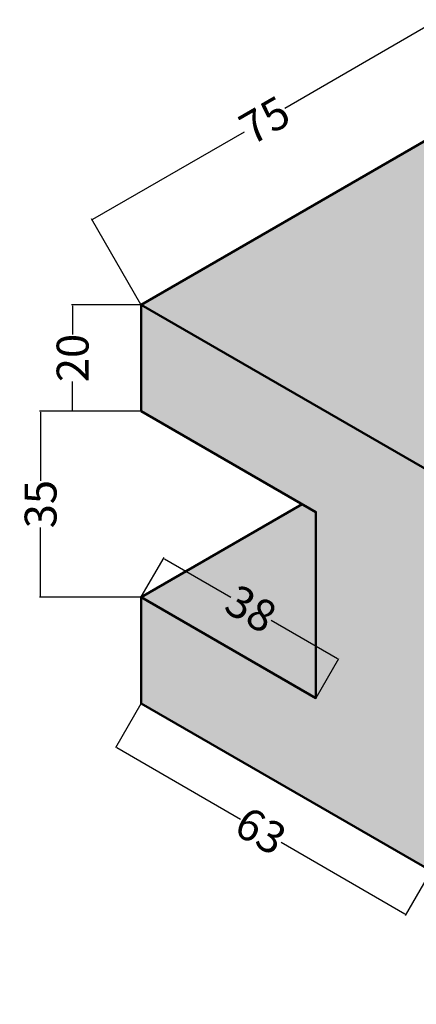
# Model space of a CAD drawing. Units: millimetres. Extents: x -24 to 183, y 0 to 191.
# Tile 1 of 1: x -23.7 to 51, y 6.1 to 191.4. Entities that reach past the tile are written whole.
import ezdxf

# ---------------------------------------------------------------- set-up
doc = ezdxf.new("R2010")
doc.units = ezdxf.units.MM
doc.header["$MEASUREMENT"] = 0
for name, color, linetype, lineweight in [('M-DIMS', 2, 'Continuous', 25), ('M-HATC', 7, 'Continuous', 18), ('M-OUTL', 7, 'Continuous', 50)]:
    doc.layers.add(name, color=color, linetype=linetype, lineweight=lineweight)
doc.styles.get("Standard").update_dxf_attribs({"font": 'arial.ttf'})
doc.dimstyles.get("Standard").update_dxf_attribs({"dimtxt": 6, "dimasz": 0.18, "dimexe": 0.18, "dimexo": 0.0625, "dimgap": 0.09, "dimtad": 0, "dimtoh": 1, "dimdec": 0, "dimzin": 0, "dimdsep": 46, "dimtxsty": 'Standard', "dimcen": 0.09, "dimadec": 0, "dimazin": 0, "dimtfac": 1, "dimtdec": 0, "dimtofl": 0, "dimtmove": 0, "dimatfit": 3, "dimfxl": 1, "dimtolj": 1, "dimtzin": 0, "dimarcsym": 0})

# ---------------------------------------------------------------- blocks, each defined once
blk = doc.blocks.new('*D3')
at = {"layer": 'Defpoints', "color": 0, "transparency": 16777216}
for p in [(54.90112838051421, 191.2180848382955), (64.142454644745, 175.211638219327), (-0.8094506390879203, 137.7116382193271)]:
    blk.add_point(p, dxfattribs=at)
at = {"layer": 'M-DIMS', "color": 0, "lineweight": -2, "transparency": 16777216}
for p, q in [((54.745243807833, 191.1280848382955), (26.22301022659634, 174.6607656022791)), ((64.111204644745, 175.2657648070636), (54.8111283805142, 191.3739694109767)), ((-9.89489233063751, 153.8080848382955), (18.62734125059916, 170.2754040743118)), ((-0.8407006390879203, 137.7657648070636), (-10.14077690331872, 153.8739694109767))]:
    blk.add_line(p, q, dxfattribs=at)
at = {"layer": 'M-DIMS', "color": 0, "transparency": 16777216}
for points in [[(54.730243807833, 191.154065600409), (54.760243807833, 191.102104076182), (54.90112838051421, 191.2180848382955)], [(-9.909892330637511, 153.834065600409), (-9.87989233063751, 153.7821040761819), (-10.05077690331871, 153.7180848382955)]]:
    blk.add_solid(points, dxfattribs=at)
at = {"layer": 'M-DIMS', "color": 0, "transparency": 16777216, "insert": (22.42517573859776, 172.4680848382955), "char_height": 6, "attachment_point": 5, "rotation": 29.999999999999993}
blk.add_mtext('\\A1;75', dxfattribs=at)
blk = doc.blocks.new('*D4')
at = {"layer": 'Defpoints', "color": 0, "transparency": 16777216}
for p in [(-0.8094506390879136, 117.7116382193271), (-19.72874656804563, 82.71163821932711), (-0.8094506390879136, 82.71163821932711)]:
    blk.add_point(p, dxfattribs=at)
at = {"layer": 'M-DIMS', "color": 0, "lineweight": -2, "transparency": 16777216}
for p, q in [((-0.8719506390879136, 117.7116382193271), (-19.90874656804564, 117.7116382193271)), ((-19.72874656804564, 117.5316382193271), (-19.72874656804564, 104.619509979218)), ((-19.72874656804563, 82.89163821932712), (-19.72874656804563, 95.80376645943628)), ((-0.8719506390879136, 82.71163821932711), (-19.90874656804563, 82.71163821932711))]:
    blk.add_line(p, q, dxfattribs=at)
at = {"layer": 'M-DIMS', "color": 0, "transparency": 16777216}
for points in [[(-19.75874656804564, 117.5316382193271), (-19.69874656804564, 117.5316382193271), (-19.72874656804564, 117.7116382193271)], [(-19.75874656804563, 82.89163821932712), (-19.69874656804563, 82.89163821932712), (-19.72874656804563, 82.71163821932711)]]:
    blk.add_solid(points, dxfattribs=at)
at = {"layer": 'M-DIMS', "color": 0, "transparency": 16777216, "insert": (-19.7287465680456, 100.2116382193271), "char_height": 6, "attachment_point": 5, "rotation": 90}
blk.add_mtext('\\A1;35', dxfattribs=at)
blk = doc.blocks.new('*D5')
at = {"layer": 'Defpoints', "color": 0, "transparency": 16777216}
for p in [(-0.8094506390879131, 82.71163821932709), (36.32281959206449, 71.02661686006039), (32.09951470472075, 63.71163821932707)]:
    blk.add_point(p, dxfattribs=at)
at = {"layer": 'M-DIMS', "color": 0, "lineweight": -2, "transparency": 16777216}
for p, q in [((-0.7782006390879133, 82.76576480706362), (3.503854248255827, 90.1825014327416)), ((3.569738820937025, 89.9366168600604), (16.06518576870042, 82.7223672011245)), ((36.1669350193833, 71.11661686006039), (23.6714880716199, 78.33086651899627)), ((32.13076470472075, 63.7657648070636), (36.41281959206449, 71.18250143274159))]:
    blk.add_line(p, q, dxfattribs=at)
at = {"layer": 'M-DIMS', "color": 0, "transparency": 16777216}
for points in [[(3.584738820937026, 89.96259762217393), (3.554738820937025, 89.91063609794686), (3.41385424825583, 90.02661686006041)], [(36.1819350193833, 71.14259762217392), (36.1519350193833, 71.09063609794686), (36.32281959206449, 71.02661686006039)]]:
    blk.add_solid(points, dxfattribs=at)
at = {"layer": 'M-DIMS', "color": 0, "transparency": 16777216, "insert": (19.86833692016016, 80.52661686006039), "char_height": 6, "attachment_point": 5, "rotation": 330}
blk.add_mtext('\\A1;38', dxfattribs=at)
blk = doc.blocks.new('*D6')
at = {"layer": 'Defpoints', "color": 0, "transparency": 16777216}
for p in [(-0.8094506390879136, 137.7116382193271), (-13.71181704573749, 117.7116382193272), (-0.8094506390879136, 117.7116382193272)]:
    blk.add_point(p, dxfattribs=at)
at = {"layer": 'M-DIMS', "color": 0, "lineweight": -2, "transparency": 16777216}
for p, q in [((-0.8719506390879136, 137.7116382193271), (-13.89181704573749, 137.7116382193271)), ((-13.71181704573749, 137.5316382193271), (-13.71181704573749, 132.1399738264213)), ((-13.71181704573749, 117.8916382193272), (-13.71181704573749, 123.283302612233)), ((-0.8719506390879136, 117.7116382193272), (-13.89181704573749, 117.7116382193272))]:
    blk.add_line(p, q, dxfattribs=at)
at = {"layer": 'M-DIMS', "color": 0, "transparency": 16777216}
for points in [[(-13.74181704573749, 137.5316382193271), (-13.68181704573749, 137.5316382193271), (-13.71181704573749, 137.7116382193271)], [(-13.74181704573748, 117.8916382193272), (-13.68181704573749, 117.8916382193272), (-13.71181704573749, 117.7116382193272)]]:
    blk.add_solid(points, dxfattribs=at)
at = {"layer": 'M-DIMS', "color": 0, "transparency": 16777216, "insert": (-13.71181704573745, 127.7116382193271), "char_height": 6, "attachment_point": 5, "rotation": 90}
blk.add_mtext('\\A1;20', dxfattribs=at)
blk = doc.blocks.new('*D7')
at = {"layer": 'Defpoints', "color": 0, "transparency": 16777216}
for p in [(-0.8094506390879097, 62.71163821932709), (53.75014979933173, 31.2116382193271), (48.99750972183936, 22.97982413502221)]:
    blk.add_point(p, dxfattribs=at)
at = {"layer": 'M-DIMS', "color": 0, "lineweight": -2, "transparency": 16777216}
for p, q in [((-0.8407006390879097, 62.65751163159055), (-5.652090716580296, 54.32393956234097)), ((-5.406206143899098, 54.38982413502217), (17.90392502424746, 40.93171363024729)), ((48.84162514915816, 23.06982413502221), (25.53149398101159, 36.5279346397971)), ((53.71889979933173, 31.15751163159057), (48.90750972183936, 22.82393956234101))]:
    blk.add_line(p, q, dxfattribs=at)
at = {"layer": 'M-DIMS', "color": 0, "transparency": 16777216}
for points in [[(-5.391206143899097, 54.41580489713571), (-5.421206143899098, 54.36384337290864), (-5.562090716580296, 54.47982413502217)], [(48.85662514915816, 23.09580489713574), (48.82662514915816, 23.04384337290867), (48.99750972183936, 22.97982413502221)]]:
    blk.add_solid(points, dxfattribs=at)
at = {"layer": 'M-DIMS', "color": 0, "transparency": 16777216, "insert": (21.71770950262953, 38.72982413502219), "char_height": 6, "attachment_point": 5, "rotation": 330}
blk.add_mtext('\\A1;63', dxfattribs=at)

msp = doc.modelspace()

# ---------------------------------------------------------------- hatches: boundary and pattern name
at = {"layer": 'M-HATC'}
h = msp.add_hatch(color=256, dxfattribs=at)
h.set_gradient(color1=(244, 238, 81), color2=(244, 238, 81), tint=1)
h.paths.add_polyline_path([(64.14245464474502, 175.211638219327), (-0.8094506390879131, 137.7116382193271), (53.75014979933173, 106.2116382193271), (118.7020550831646, 143.7116382193271)])
edge = h.paths.add_edge_path()
edge.add_line((95.31936918098478, 130.2116382193271), (77.13283570151161, 119.7116382193271))
edge.add_spline(control_points=[(77.13283570151158, 119.7116382193271), (89.17924906810929, 107.2566382193724), (101.2256624347508, 94.80163821937239)], knot_values=[5.356194490192345, 5.356194490192345, 5.356194490192345, 6.356194490188707, 6.356194490192345, 6.356194490192345], weights=[1, 1, 1], degree=2, periodic=0)
edge.add_spline(control_points=[(101.2256624347947, 94.80163821932707), (110.3189291745312, 100.051638219327), (119.4121959142679, 105.301638219327)], knot_values=[6.356194490188707, 6.356194490192345, 6.356194490192345, 7.356194490192345, 7.356194490192345, 7.356194490192345], weights=[1, 1, 1], degree=2, periodic=0)
edge.add_line((119.4121959142679, 105.3016382193271), (95.31936918098478, 130.2116382193271))
edge = h.paths.add_edge_path()
edge.add_spline(control_points=[(150.7449950231889, 106.2116382193271), (134.7235250531767, 115.4616382193271), (118.7020550831646, 124.7116382193271)], knot_values=[3.356194490192345, 3.356194490192345, 3.356194490192345, 4.178416712414569, 4.178416712414569, 4.178416712414569], weights=[1, 1, 1], degree=2, periodic=0)
edge.add_spline(control_points=[(118.7020550831646, 124.7116382193271), (115.2379534680269, 126.7116382193271), (111.7738518528891, 128.7116382193271)], knot_values=[4.178416712414569, 4.178416712414569, 4.178416712414569, 4.356194490192345, 4.356194490192345, 4.356194490192345], weights=[1, 1, 1], degree=2, periodic=0)
edge.add_spline(control_points=[(111.7738518528891, 128.7116382193271), (106.960071285434, 125.9324007128871), (102.1462907179789, 123.1531632064471)], knot_values=[4.356194490192345, 4.356194490192345, 4.356194490192345, 5.356194490192345, 5.356194490192345, 5.356194490192345], weights=[1, 1, 1], degree=2, periodic=0)
edge.add_line((102.1462907179789, 123.1531632064471), (119.4121959142679, 105.301638219327))
edge.add_spline(control_points=[(119.4121959142679, 105.301638219327), (126.8513541327762, 101.006638219327), (134.2905123512845, 96.71163821932709)], knot_values=[7.356194490192345, 7.356194490192345, 7.356194490192345, 8.356194490192346, 8.356194490192346, 8.356194490192346], weights=[1, 1, 1], degree=2, periodic=0)
edge.add_spline(control_points=[(134.2905123512845, 96.71163821932709), (158.0953395036126, 82.96791485491796), (161.6862132372617, 53.72180942535438), (165.2770869709107, 24.47570399579081), (142.5556009483879, 29.39608484008592)], knot_values=[8.356194490192346, 8.356194490192346, 8.356194490192346, 9.775566349411587, 9.775566349411587, 11.19493820863083, 11.19493820863083, 11.19493820863083], weights=[1, 0.7585665602715825, 1, 0.7585665602715825, 1], degree=2, periodic=0)
edge.add_spline(control_points=[(153.8864302935499, 30.77051272237281), (162.1136716295021, 35.52051272237281), (170.3409129654543, 40.2705127223728)], knot_values=[0, 0, 0, 1, 1, 1], weights=[1, 1, 1], degree=2, periodic=0)
edge.add_spline(control_points=[(170.3409129654543, 40.2705127223728), (183.4344867248955, 47.83009105704043), (176.3482956693094, 71.67543553482938), (169.2621046137232, 95.5207800126183), (150.7449950231889, 106.2116382193271)], knot_values=[1, 1, 1, 2.178097245096171, 2.178097245096171, 3.356194490192345, 3.356194490192345, 3.356194490192345], weights=[1, 0.831469612302545, 1, 0.831469612302545, 1], degree=2, periodic=0)
edge = h.paths.add_edge_path(flags=17)
edge.add_spline(control_points=[(134.2905123512845, 96.71163821932709), (126.8513541327762, 101.006638219327), (119.4121959142679, 105.301638219327)], knot_values=[7.356194490192345, 7.356194490192345, 7.356194490192345, 8.356194490192346, 8.356194490192346, 8.356194490192346], weights=[1, 1, 1], degree=2, periodic=0)
edge.add_line((119.4121959142679, 105.301638219327), (119.4121959142679, 84.07281383496964))
edge.add_spline(control_points=[(119.4121959142679, 84.07281383496964), (123.0724490086632, 81.4513939238958), (126.4903518736498, 77.88262675949477)], knot_values=[2.966768687208849, 2.966768687208849, 2.966768687208849, 3.231438789490306, 3.231438789490306, 3.231438789490306], weights=[0.9680864183363699, 0.938243390584542, 0.9254123758008628], degree=2, periodic=0)
edge.add_ellipse((134.2905123512845, 64.71163821932709), major_axis=(7.654655446197426, -13.25825214724777), ratio=0.5773502691896262, start_angle=359.3650130620468, end_angle=540.634986937953, ccw=False)
edge.add_spline(control_points=[(141.7968427812057, 51.37100682201758), (145.5119247027769, 38.61436904653682), (142.5556009483879, 29.39608484008592)], knot_values=[1.485548755374229, 1.485548755374229, 1.485548755374229, 2.169061485720957, 2.169061485720957, 2.169061485720957], weights=[0.9974346422091759, 0.9011559533067647, 0.9183363162707197], degree=2, periodic=0)
edge.add_spline(control_points=[(142.5556009483879, 29.39608484008592), (165.2770869709107, 24.47570399579081), (161.6862132372617, 53.72180942535438), (158.0953395036126, 82.96791485491796), (134.2905123512845, 96.71163821932709)], knot_values=[8.356194490192342, 8.356194490192342, 8.356194490192342, 9.775566349411587, 9.775566349411587, 11.19493820863083, 11.19493820863083, 11.19493820863083], weights=[1, 0.7585665602715825, 1, 0.7585665602715825, 1], degree=2, periodic=0)
edge = h.paths.add_edge_path()
edge.add_spline(control_points=[(119.4121959142679, 105.301638219327), (110.3189291745312, 100.051638219327), (101.2256624347947, 94.80163821932707)], knot_values=[6.356194490188707, 6.356194490188707, 6.356194490188707, 7.356194490188707, 7.356194490188707, 7.356194490192345], weights=[1, 1, 1], degree=2, periodic=0)
edge.add_spline(control_points=[(101.2256624347947, 94.80163821932709), (108.664820653303, 90.5066382193271), (116.1039788718113, 86.21163821932711)], knot_values=[3.356194490192346, 3.356194490192346, 3.356194490192346, 3.737972267970123, 3.737972267970123, 3.737972267970123], weights=[1, 1, 1], degree=2, periodic=0)
edge.add_spline(control_points=[(116.1039788718113, 86.21163821932711), (117.7640226821475, 85.25321147856292), (119.4121959142679, 84.07281383496964)], knot_values=[3.231438789490306, 3.231438789490306, 3.231438789490306, 3.356194490192346, 3.356194490192346, 3.356194490192346], weights=[1, 0.9821533182474542, 0.9680864183363699], degree=2, periodic=0)
edge.add_line((119.4121959142679, 84.07281383496965), (119.4121959142679, 105.301638219327))
h.paths.add_polyline_path([(-0.8094506390879131, 137.7116382193271), (-0.8094506390879131, 117.7116382193271), (32.09951470472076, 98.71163821932709), (32.09951470472076, 63.71163821932707), (-0.8094506390879131, 82.71163821932709), (-0.8094506390879062, 62.71163821932709), (53.75014979933173, 31.21163821932709), (53.75014979933173, 106.2116382193271)])
h.paths.add_polyline_path([(32.09951470472076, 98.71163821932709), (29.50143849336745, 100.2116382193271), (-0.8094506390879203, 82.71163821932709), (32.09951470472076, 63.71163821932708)])
edge = h.paths.add_edge_path()
edge.add_spline(control_points=[(99.64949619990696, 57.21163821932711), (99.64949619990696, 66.96163821932711), (99.64949619990696, 76.71163821932711)], knot_values=[5.141592653589794, 5.141592653589794, 5.141592653589794, 5.446280153589794, 5.446280153589794, 5.446280153589794], weights=[1, 1, 1], degree=2, periodic=0)
edge.add_line((99.64949619990699, 76.7116382193271), (60.67835302960723, 99.2116382193271))
edge.add_spline(control_points=[(60.67835302960723, 99.2116382193271), (60.67835302960723, 67.2116382193271), (60.67835302960723, 35.2116382193271)], knot_values=[0, 0, 0, 1, 1, 1], weights=[1, 1, 1], degree=2, periodic=0)
edge.add_spline(control_points=[(60.67835302960723, 35.2116382193271), (80.16392461475712, 23.9616382193271), (99.64949619990699, 12.71163821932711)], knot_values=[1, 1, 1, 2, 2, 2], weights=[1, 1, 1], degree=2, periodic=0)
edge.add_spline(control_points=[(99.64949619990699, 12.7116382193271), (99.64949619990699, 22.4616382193271), (99.64949619990699, 32.2116382193271)], knot_values=[5.836905153589794, 5.836905153589794, 5.836905153589794, 6.141592653589794, 6.141592653589794, 6.141592653589794], weights=[1, 1, 1], degree=2, periodic=0)
edge.add_ellipse((99.64949619990699, 44.7116382193271), major_axis=(7.654655446197426, -13.25825214724777), ratio=0.5773502691896261, start_angle=150, end_angle=330, ccw=False)
edge = h.paths.add_edge_path(flags=17)
edge.add_spline(control_points=[(77.13283570151158, 119.7116382193271), (77.13283570151158, 114.2116382193271), (77.13283570151158, 108.711638219327)], knot_values=[4.356194490192345, 4.356194490192345, 4.356194490192345, 5.356194490192345, 5.356194490192345, 5.356194490192345], weights=[1, 1, 1], degree=2, periodic=0)
edge.add_spline(control_points=[(77.13283570151158, 108.711638219327), (89.17924906815313, 101.7566382193271), (101.2256624347947, 94.80163821932709)], knot_values=[3.737972267970123, 3.737972267970123, 3.737972267970123, 4.356194490192345, 4.356194490192345, 4.356194490192345], weights=[1, 1, 1], degree=2, periodic=0)
edge.add_spline(control_points=[(101.2256624347508, 94.80163821937239), (89.17924906810929, 107.2566382193724), (77.13283570151158, 119.7116382193271)], knot_values=[5.356194490192345, 5.356194490192345, 5.356194490195983, 6.356194490192345, 6.356194490192345, 6.356194490192345], weights=[1, 1, 1], degree=2, periodic=0)
edge = h.paths.add_edge_path()
edge.add_spline(control_points=[(119.2454141421726, 10.77051272237291), (121.8252656817894, 12.25999070323999), (123.649496199907, 14.85523175877608), (131.649496199907, 26.23642960525908), (123.649496199907, 46.8552317587761), (115.649496199907, 67.4740339122931), (99.64949619990696, 76.71163821932711)], knot_values=[2.780860556892677, 2.780860556892677, 2.780860556892677, 3.047197551196599, 3.047197551196599, 4.094395102393195, 4.094395102393195, 5.141592653589794, 5.141592653589794, 5.141592653589794], weights=[0.9491840326991366, 0.9659258262890693, 1, 0.8660254037844385, 1, 0.8660254037844385, 1], degree=2, periodic=0)
edge.add_spline(control_points=[(99.64949619990696, 76.71163821932711), (99.64949619990696, 66.96163821932711), (99.64949619990696, 57.21163821932711)], knot_values=[5.141592653589794, 5.141592653589794, 5.141592653589794, 5.446280153589794, 5.446280153589794, 5.446280153589794], weights=[1, 1, 1], degree=2, periodic=0)
edge.add_ellipse((99.64949619990699, 44.7116382193271), major_axis=(7.654655446197426, -13.25825214724777), ratio=0.5773502691896261, start_angle=330, end_angle=509.9999999999999, ccw=False)
edge.add_spline(control_points=[(99.64949619990699, 32.2116382193271), (99.64949619990699, 22.4616382193271), (99.64949619990699, 12.7116382193271)], knot_values=[5.836905153589794, 5.836905153589794, 5.836905153589794, 6.141592653589794, 6.141592653589794, 6.141592653589794], weights=[1, 1, 1], degree=2, periodic=0)
edge.add_spline(control_points=[(99.64949619990699, 12.71163821932711), (111.1285191633359, 6.084221221357497), (119.2454141421726, 10.77051272237291)], knot_values=[2, 2, 2, 2.780860556892677, 2.780860556892677, 2.780860556892677], weights=[1, 0.9000995774953693, 0.9491840326991366], degree=2, periodic=0)
edge = h.paths.add_edge_path()
edge.add_line((118.7020550831646, 143.7116382193271), (95.31936918098478, 130.2116382193271))
edge.add_line((95.31936918098478, 130.2116382193271), (102.1462907179789, 123.1531632064471))
edge.add_spline(control_points=[(102.1462907179789, 123.1531632064471), (106.960071285434, 125.9324007128871), (111.7738518528891, 128.7116382193271)], knot_values=[4.356194490192345, 4.356194490192345, 4.356194490192345, 5.356194490192345, 5.356194490192345, 5.356194490192345], weights=[1, 1, 1], degree=2, periodic=0)
edge.add_spline(control_points=[(111.7738518528891, 128.7116382193271), (115.2379534680269, 126.7116382193271), (118.7020550831646, 124.7116382193271)], knot_values=[4.178416712414568, 4.178416712414568, 4.178416712414568, 4.356194490192344, 4.356194490192344, 4.356194490192344], weights=[1, 1, 1], degree=2, periodic=0)
edge.add_line((118.7020550831646, 124.7116382193271), (118.7020550831646, 143.7116382193271))

# ---------------------------------------------------------------- linework, layer by layer
at = {"layer": 'M-OUTL'}
for points in [[(53.75014979933173, 106.2116382193271), (-0.8094506390879131, 137.7116382193271), (64.14245464474502, 175.211638219327), (118.7020550831646, 143.7116382193271), (118.7020550831646, 124.7116382193271)], [(-0.8094506390879131, 137.7116382193271), (-0.8094506390879131, 117.7116382193271), (32.09951470472076, 98.71163821932709), (32.09951470472076, 63.71163821932708), (-0.8094506390879131, 82.71163821932709), (29.50143849336745, 100.2116382193271)], [(53.75014979933173, 31.2116382193271), (-0.8094506390879131, 62.71163821932709), (-0.8094506390879131, 82.71163821932709)]]:
    msp.add_lwpolyline(points, dxfattribs=at)

# ---------------------------------------------------------------- dimensions: what is measured, and where the dimension line sits
at = {"layer": 'M-DIMS'}
for p1, p2, distance, picture, middle in [((-0.8094506390879131, 137.7116382193271), (64.14245464474502, 175.211638219327), 18.48265252846167, '*D3', (22.42517573859776, 172.4680848382955)), ((-0.8094506390879131, 137.7116382193271), (-0.8094506390879131, 117.7116382193271), -12.902366406649577, '*D6', (-13.71181704573745, 127.7116382193271)), ((-0.8094506390879131, 117.7116382193271), (-0.8094506390879131, 82.71163821932709), -18.919295928957716, '*D4', (-19.7287465680456, 100.2116382193271)), ((-0.8094506390879131, 82.71163821932709), (32.09951470472076, 63.71163821932708), 8.446609774687472, '*D5', (19.86833692016016, 80.52661686006039)), ((-0.8094506390879131, 62.71163821932709), (53.75014979933173, 31.2116382193271), -9.505280154984762, '*D7', (21.71770950262953, 38.72982413502219))]:
    dim = msp.add_aligned_dim(p1=p1, p2=p2, distance=distance, dimstyle='Standard', override={"dimclrd": 0, "dimclre": 0, "dimclrt": 0}, dxfattribs=at)
    dim.commit()
    dim.dimension.update_dxf_attribs({"geometry": picture, "text_midpoint": middle})

doc.saveas('drawing.dxf')
